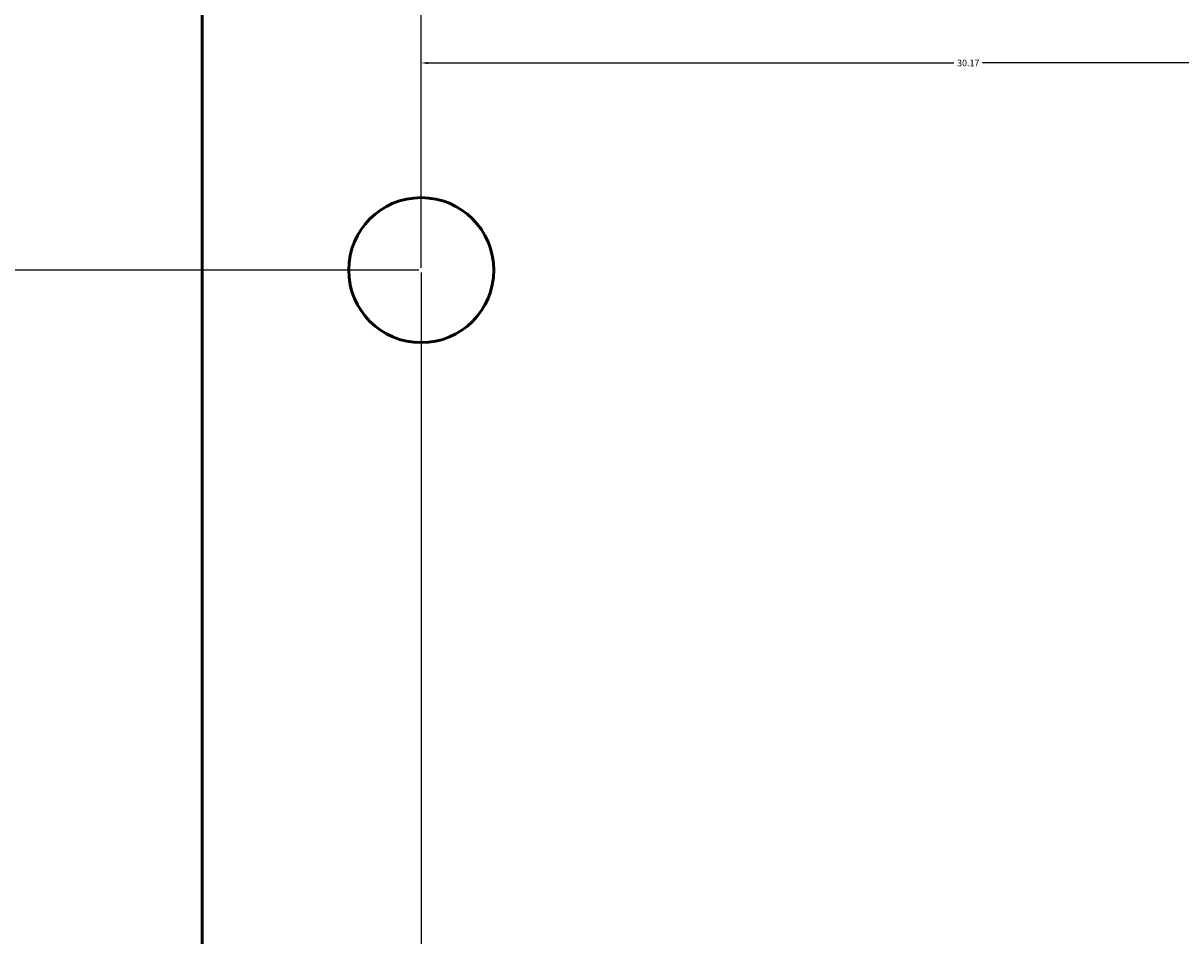
# Model space of a CAD drawing. Units: inches. Extents: x -14 to 108, y -9 to 83.
# Tile 4 of 13: x 6 to 38, y 19 to 44. Entities that reach past the tile are written whole.
import ezdxf

# ---------------------------------------------------------------- set-up
doc = ezdxf.new("R2010")
doc.units = ezdxf.units.IN
doc.header["$MEASUREMENT"] = 0
doc.layers.add('M-DIMS', color=2, linetype='Continuous', lineweight=18)
doc.layers.add('M-OUTL', color=7, linetype='Continuous', lineweight=50)
doc.styles.get("Standard").update_dxf_attribs({"font": 'arial.ttf'})
doc.dimstyles.get("Standard").update_dxf_attribs({"dimtxt": 0.18, "dimasz": 0.18, "dimexe": 0.18, "dimexo": 0.0625, "dimgap": 0.09, "dimtad": 0, "dimtih": 1, "dimtoh": 1, "dimzin": 0, "dimdsep": 46, "dimtxsty": 'Standard', "dimcen": 0.09, "dimadec": 0, "dimazin": 0, "dimtfac": 1, "dimtofl": 0, "dimtmove": 0, "dimatfit": 3, "dimfxl": 1, "dimtolj": 1, "dimtzin": 0, "dimarcsym": 0})

# ---------------------------------------------------------------- blocks, each defined once
blk = doc.blocks.new('SLOT-VERTICAL')
blk.add_lwpolyline([(4.933, 40.458), (4.933, 1.021)])
blk = doc.blocks.new('HOLE-D4')
blk.add_circle((2, 2), 2)
blk = doc.blocks.new('*D7')
at = {"layer": 'Defpoints', "color": 0, "transparency": 16777216}
for p in [(47.098, 37.119), (5.951, 18.227), (47.098, -8.596)]:
    blk.add_point(p, dxfattribs=at)
at = {"layer": 'M-DIMS', "color": 0, "lineweight": -2, "transparency": 16777216}
for p, q in [((47.098, 37.057), (47.098, -8.776)), ((5.951, 18.165), (5.951, -8.776)), ((6.131, -8.596), (26.126, -8.596)), ((46.918, -8.596), (26.922, -8.596))]:
    blk.add_line(p, q, dxfattribs=at)
at = {"layer": 'M-DIMS', "color": 0, "transparency": 16777216}
for points in [[(6.131, -8.566), (6.131, -8.626), (5.951, -8.596)], [(46.918, -8.566), (46.918, -8.626), (47.098, -8.596)]]:
    blk.add_solid(points, dxfattribs=at)
at = {"layer": 'M-DIMS', "color": 0, "transparency": 16777216, "insert": (26.524, -8.596), "char_height": 0.18, "attachment_point": 5}
blk.add_mtext('\\A1;41.15', dxfattribs=at)
blk = doc.blocks.new('*D13')
at = {"layer": 'Defpoints', "color": 0, "transparency": 16777216}
for p in [(26.462, 82.834), (26.462, 55.756), (16.928, 37.119)]:
    blk.add_point(p, dxfattribs=at)
at = {"layer": 'M-DIMS', "color": 0, "lineweight": -2, "transparency": 16777216}
for p, q in [((16.928, 37.182), (16.928, 83.014)), ((26.462, 55.818), (26.462, 83.014)), ((17.108, 82.834), (21.301, 82.834)), ((26.282, 82.834), (22.088, 82.834))]:
    blk.add_line(p, q, dxfattribs=at)
at = {"layer": 'M-DIMS', "color": 0, "transparency": 16777216}
for points in [[(17.108, 82.864), (17.108, 82.804), (16.928, 82.834)], [(26.282, 82.864), (26.282, 82.804), (26.462, 82.834)]]:
    blk.add_solid(points, dxfattribs=at)
at = {"layer": 'M-DIMS', "color": 0, "transparency": 16777216, "insert": (21.695, 82.834), "char_height": 0.18, "attachment_point": 5}
blk.add_mtext('\\A1;9.534', dxfattribs=at)
blk = doc.blocks.new('*D14')
at = {"layer": 'Defpoints', "color": 0, "transparency": 16777216}
for p in [(47.098, 42.834), (16.928, 37.119), (47.098, 37.119)]:
    blk.add_point(p, dxfattribs=at)
at = {"layer": 'M-DIMS', "color": 0, "lineweight": -2, "transparency": 16777216}
for p, q in [((16.928, 37.182), (16.928, 43.014)), ((17.108, 42.834), (31.619, 42.834)), ((46.918, 42.834), (32.407, 42.834)), ((47.098, 37.182), (47.098, 43.014))]:
    blk.add_line(p, q, dxfattribs=at)
at = {"layer": 'M-DIMS', "color": 0, "transparency": 16777216}
for points in [[(17.108, 42.864), (17.108, 42.804), (16.928, 42.834)], [(46.918, 42.864), (46.918, 42.804), (47.098, 42.834)]]:
    blk.add_solid(points, dxfattribs=at)
at = {"layer": 'M-DIMS', "color": 0, "transparency": 16777216, "insert": (32.013, 42.834), "char_height": 0.18, "attachment_point": 5}
blk.add_mtext('\\A1;30.17', dxfattribs=at)
blk = doc.blocks.new('*D16')
at = {"layer": 'Defpoints', "color": 0, "transparency": 16777216}
for p in [(16.928, 37.119), (27.381, 15.402), (27.381, -8.596)]:
    blk.add_point(p, dxfattribs=at)
at = {"layer": 'M-DIMS', "color": 0, "lineweight": -2, "transparency": 16777216}
for p, q in [((16.928, 37.057), (16.928, -8.776)), ((27.381, 15.34), (27.381, -8.776)), ((17.108, -8.596), (21.699, -8.596)), ((27.201, -8.596), (22.61, -8.596))]:
    blk.add_line(p, q, dxfattribs=at)
at = {"layer": 'M-DIMS', "color": 0, "transparency": 16777216}
for points in [[(17.108, -8.566), (17.108, -8.626), (16.928, -8.596)], [(27.201, -8.566), (27.201, -8.626), (27.381, -8.596)]]:
    blk.add_solid(points, dxfattribs=at)
at = {"layer": 'M-DIMS', "color": 0, "transparency": 16777216, "insert": (22.154, -8.596), "char_height": 0.18, "attachment_point": 5}
blk.add_mtext('\\A1;10.453', dxfattribs=at)
blk = doc.blocks.new('*D18')
at = {"layer": 'Defpoints', "color": 0, "transparency": 16777216}
for p in [(-13.617, 55.756), (26.462, 55.756), (16.928, 37.119)]:
    blk.add_point(p, dxfattribs=at)
at = {"layer": 'M-DIMS', "color": 0, "lineweight": -2, "transparency": 16777216}
for p, q in [((26.399, 55.756), (-13.797, 55.756)), ((-13.617, 55.576), (-13.617, 46.619)), ((-13.617, 37.299), (-13.617, 46.256)), ((16.865, 37.119), (-13.797, 37.119))]:
    blk.add_line(p, q, dxfattribs=at)
at = {"layer": 'M-DIMS', "color": 0, "transparency": 16777216}
for points in [[(-13.647, 55.576), (-13.587, 55.576), (-13.617, 55.756)], [(-13.647, 37.299), (-13.587, 37.299), (-13.617, 37.119)]]:
    blk.add_solid(points, dxfattribs=at)
at = {"layer": 'M-DIMS', "color": 0, "transparency": 16777216, "insert": (-13.617, 46.437), "char_height": 0.18, "attachment_point": 5}
blk.add_mtext('\\A1;18.636', dxfattribs=at)
blk = doc.blocks.new('*D19')
at = {"layer": 'Defpoints', "color": 0, "transparency": 16777216}
for p in [(-13.617, 37.119), (16.928, 37.119), (27.381, 15.402)]:
    blk.add_point(p, dxfattribs=at)
at = {"layer": 'M-DIMS', "color": 0, "lineweight": -2, "transparency": 16777216}
for p, q in [((16.865, 37.119), (-13.797, 37.119)), ((-13.617, 36.939), (-13.617, 26.441)), ((-13.617, 15.582), (-13.617, 26.08)), ((27.318, 15.402), (-13.797, 15.402))]:
    blk.add_line(p, q, dxfattribs=at)
at = {"layer": 'M-DIMS', "color": 0, "transparency": 16777216}
for points in [[(-13.647, 36.939), (-13.587, 36.939), (-13.617, 37.119)], [(-13.647, 15.582), (-13.587, 15.582), (-13.617, 15.402)]]:
    blk.add_solid(points, dxfattribs=at)
at = {"layer": 'M-DIMS', "color": 0, "transparency": 16777216, "insert": (-13.617, 26.261), "char_height": 0.18, "attachment_point": 5}
blk.add_mtext('\\A1;21.717', dxfattribs=at)

msp = doc.modelspace()

# ---------------------------------------------------------------- block references
at = {"layer": 'M-OUTL'}
for name, p in [('SLOT-VERTICAL', (5.9511, 17.206)), ('HOLE-D4', (14.928, 35.119))]:
    msp.add_blockref(name, p, dxfattribs=at)

# ---------------------------------------------------------------- dimensions: what is measured, and where the dimension line sits
at = {"layer": 'M-DIMS'}
for base, p1, p2, override, picture, middle in [((26.4616, 82.8343), (16.9278, 37.1193), (26.4616, 55.7556), {"dimdec": 3, "dimlfac": 1, "dimrnd": 0, "dimzin": 0, "dimdsep": 46, "dimlunit": 2}, '*D13', (21.6947, 82.8343)), ((47.0979, -8.5957), (5.9508, 18.2274), (47.0979, 37.1193), {"dimdec": 2, "dimlfac": 1, "dimrnd": 0, "dimzin": 0, "dimdsep": 46, "dimlunit": 2}, '*D7', (26.5244, -8.5957)), ((27.3809, -8.5957), (16.9278, 37.1193), (27.3809, 15.4023), {"dimdec": 3, "dimlfac": 1, "dimrnd": 0, "dimzin": 0, "dimdsep": 46, "dimlunit": 2}, '*D16', (22.1543, -8.5957))]:
    dim = msp.add_linear_dim(base=base, p1=p1, p2=p2, dimstyle='Standard', override=override, dxfattribs=at)
    dim.commit()
    dim.dimension.update_dxf_attribs({"geometry": picture, "text_midpoint": middle})
for base, p1, p2, angle, override, picture, middle in [((-13.6171, 55.7556), (16.9278, 37.1193), (26.4616, 55.7556), 90, {"dimdec": 3, "dimlfac": 1, "dimrnd": 0, "dimzin": 0, "dimdsep": 46, "dimlunit": 2}, '*D18', (-13.6171, 46.4375)), ((47.0979, 42.8343), (16.9278, 37.1193), (47.0979, 37.1193), 0, {"dimdec": 2, "dimlfac": 1, "dimrnd": 0, "dimzin": 0, "dimdsep": 46, "dimlunit": 2}, '*D14', (32.0129, 42.8343)), ((-13.6171, 37.1193), (27.3809, 15.4023), (16.9278, 37.1193), 90, {"dimdec": 3, "dimlfac": 1, "dimrnd": 0, "dimzin": 0, "dimdsep": 46, "dimlunit": 2}, '*D19', (-13.6171, 26.2608))]:
    dim = msp.add_linear_dim(base=base, p1=p1, p2=p2, angle=angle, dimstyle='Standard', override=override, dxfattribs=at)
    dim.commit()
    dim.dimension.update_dxf_attribs({"geometry": picture, "text_midpoint": middle})

doc.saveas('drawing.dxf')
